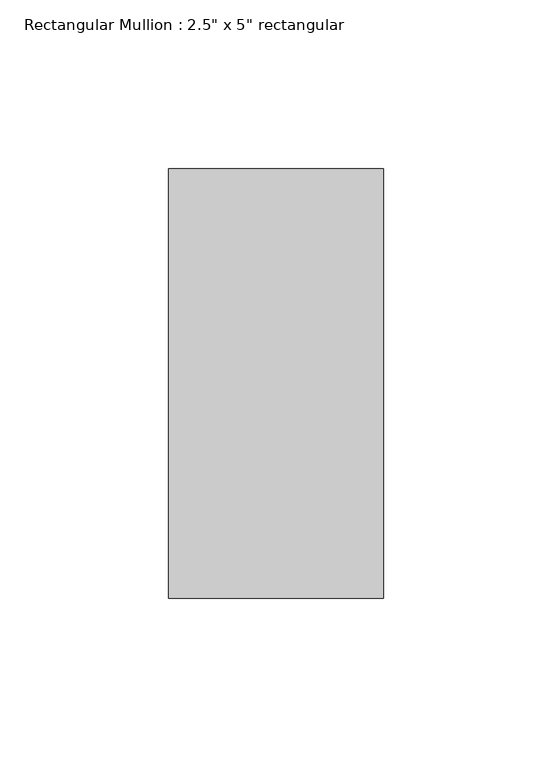
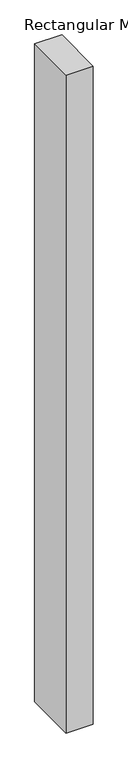
"""IFC4 building model written with IfcOpenShell, lengths in millimetres: member geometry."""

from ifc_helpers import new_model, si_unit, frame, origin, place, context, project, spatial, polyline, outline, extrude, source, transform, mapped, element, save


def member_a27facc5(model_context):
    return source(origin(), model_context, "Body", "SweptSolid", [
        extrude(outline(polyline([(31.75, 63.5), (31.75, -63.5), (-31.75, -63.5), (-31.75, 63.5), (31.75, 63.5)])), frame((0.0, 0.0, -1624.4964589), z_axis=(0.0, 0.0, 1.0), x_axis=(1.0, 0.0, 0.0)), (0.0, 0.0, 1.0), 1624.4964589),
    ])


if __name__ == "__main__":
    model = new_model("IFC4")
    model_context = context("Model", 3, world=origin())
    ifc_project = project(units=[si_unit("LENGTHUNIT", "METRE", prefix="MILLI")], contexts=[model_context])
    site = spatial("IfcSite", under=ifc_project)
    building = spatial("IfcBuilding", under=site)
    placement = place(None, origin())
    member_shape = member_a27facc5(model_context)
    element("IfcMember", 1, ObjectType="Rectangular Mullion : 2.5\" x 5\" rectangular", at=placement, inside=building, context=model_context, shape_type="MappedRepresentation", body=[
        mapped(member_shape, transform((0.0, 0.0, 0.0), x_axis=(1.0, 0.0, 0.0), y_axis=(0.0, 1.0, 0.0), z_axis=(0.0, 0.0, 1.0))),
    ])
    save(model, "model.ifc")

# Revit data of these elements
# Type "Rectangular Mullion : 2.5\" x 5\" rectangular"
#   built-in parameter 1007304 = 0.416667 (stored number, unit not read)
#   built-in parameter 1007301 = 0.104167 (stored number, unit not read)
#   built-in parameter 1007300 = 0.104167 (stored number, unit not read)
# Element 1 (IfcMember, "Rectangular Mullion : 2.5\" x 5\" rectangular")
#   Materials on its faces: "Aluminum"
# Materials
#   "Aluminum": class "Metal", colour RGB 247 247 247, transparency 0, Description = "Aluminum 6061", Cost = 0
